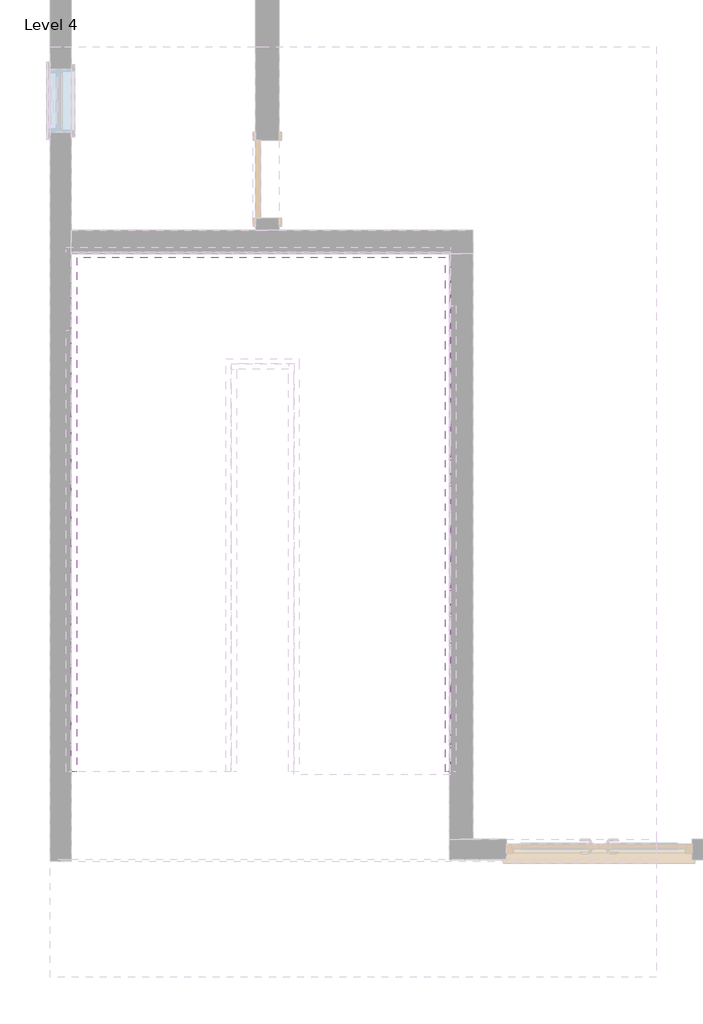
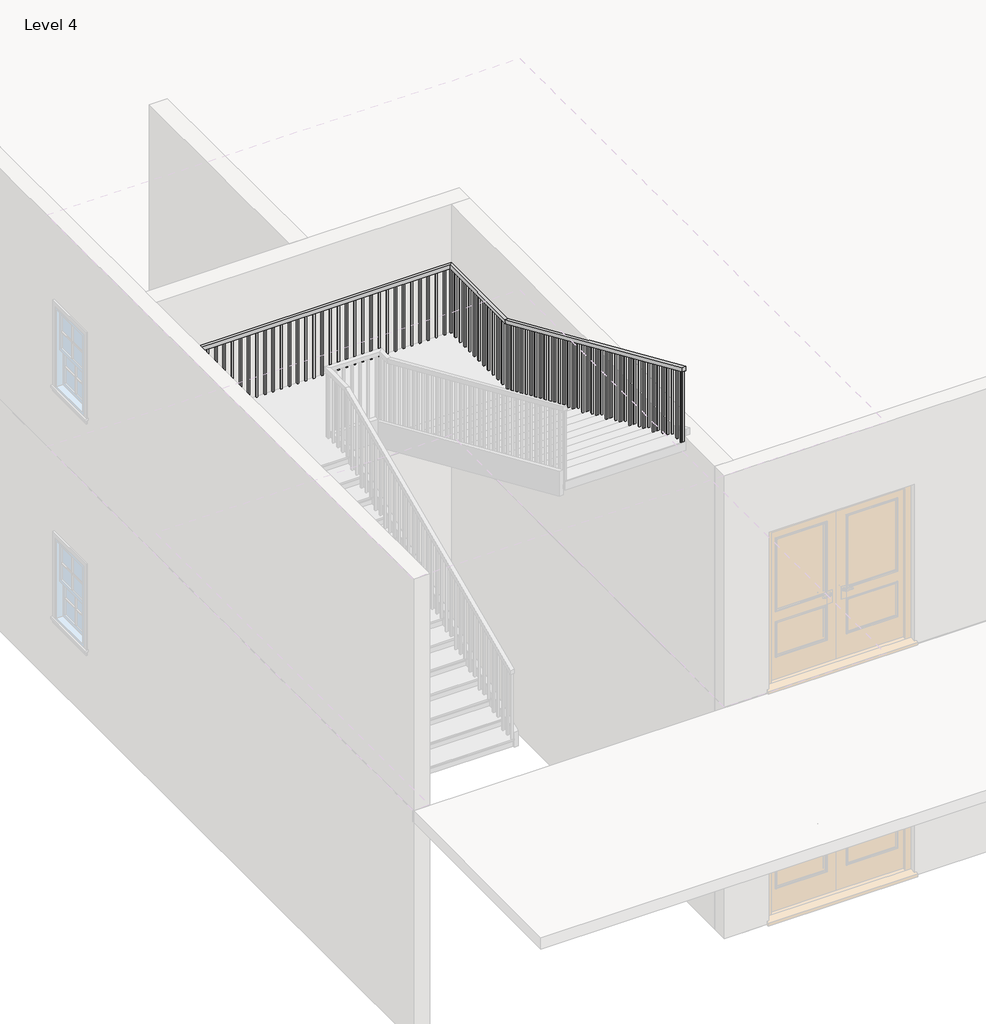
# One storey, part 4 of 5: 1 railing.
"""IFC4 building model written with IfcOpenShell, lengths in millimetres."""

from ifc_helpers import new_model, si_unit, frame, origin, place, context, project, spatial, polyline, outline, extrude, faceted_brep, element, save

model = new_model("IFC4")

# Units and contexts
model_context = context("Model", 3, world=origin())
ifc_project = project(units=[si_unit("LENGTHUNIT", "METRE", prefix="MILLI")], contexts=[model_context])

# Site, building, storey
site = spatial("IfcSite", under=ifc_project)
building = spatial("IfcBuilding", under=site)
storey = spatial("IfcBuildingStorey", under=building, Name="Level 4", Elevation=9144.0)

# Railing
placement = place(None, origin())
element("IfcRailing", 1, ObjectType="Handrail - Rectangular", at=placement, inside=storey, context=model_context, shape_type="SolidModel", body=[
    faceted_brep([(-7554.4415084, -6973.0610642, 12913.36), (-7554.4415084, -6973.0610642, 12857.8599828), (-7503.6415084, -6973.0610642, 12857.8599828), (-7503.6415084, -6973.0610642, 12913.36), (-7554.4415084, -3417.0610642, 14478.0), (-7554.4415084, -3406.3792071, 14427.2), (-7503.6415084, -3406.3792071, 14427.2), (-7503.6415084, -3417.0610642, 14478.0), (-7554.4415084, -1928.4217109, 14478.0), (-7554.4415084, -1928.4217109, 14427.2), (-7503.6415084, -1979.2217109, 14427.2), (-7503.6415084, -1979.2217109, 14478.0), (-3866.3290366, -1928.4217109, 14478.0), (-3866.3290366, -1928.4217109, 14427.2), (-3917.1290366, -1979.2217109, 14427.2), (-3917.1290366, -1979.2217109, 14478.0), (-3866.3290366, -3163.0610642, 14478.0), (-3866.3290366, -3173.7429214, 14427.2), (-3917.1290366, -3173.7429214, 14427.2), (-3917.1290366, -3163.0610642, 14478.0), (-3866.3290366, -6973.0610642, 16154.4), (-3917.1290366, -6973.0610642, 16154.4), (-3917.1290366, -6973.0610642, 16098.8999828), (-3866.3290366, -6973.0610642, 16098.8999828)], [[[0, 1, 2, 3]], [[1, 0, 4, 5]], [[2, 1, 5, 6]], [[3, 2, 6, 7]], [[0, 3, 7, 4]], [[5, 4, 8, 9]], [[6, 5, 9, 10]], [[7, 6, 10, 11]], [[4, 7, 11, 8]], [[9, 8, 12, 13]], [[10, 9, 13, 14]], [[11, 10, 14, 15]], [[8, 11, 15, 12]], [[13, 12, 16, 17]], [[14, 13, 17, 18]], [[15, 14, 18, 19]], [[12, 15, 19, 16]], [[20, 21, 22, 23]], [[17, 16, 20, 23]], [[18, 17, 23, 22]], [[19, 18, 22, 21]], [[16, 19, 21, 20]]]),
    extrude(outline(polyline([(-6922.6967109, 16076.7396674), (-6922.6967109, 15128.24), (-6941.7467109, 15128.24), (-6941.7467109, 16085.1216674), (-6922.6967109, 16076.7396674)])), frame((-3901.2540366, 0.0, 0.0), z_axis=(1.0, 0.0, 0.0), x_axis=(0.0, 1.0, 0.0)), (0.0, 0.0, 1.0), 19.05),
    extrude(outline(polyline([(-6821.0967109, 16032.0356674), (-6821.0967109, 15128.24), (-6840.1467109, 15128.24), (-6840.1467109, 16040.4176674), (-6821.0967109, 16032.0356674)])), frame((-3901.2540366, 0.0, 0.0), z_axis=(1.0, 0.0, 0.0), x_axis=(0.0, 1.0, 0.0)), (0.0, 0.0, 1.0), 19.05),
    extrude(outline(polyline([(-6719.4967109, 15987.3316674), (-6719.4967109, 15128.24), (-6738.5467109, 15128.24), (-6738.5467109, 15995.7136674), (-6719.4967109, 15987.3316674)])), frame((-3901.2540366, 0.0, 0.0), z_axis=(1.0, 0.0, 0.0), x_axis=(0.0, 1.0, 0.0)), (0.0, 0.0, 1.0), 19.05),
    extrude(outline(polyline([(-6617.8967109, 15942.6276674), (-6617.8967109, 15016.48), (-6636.9467109, 15016.48), (-6636.9467109, 15951.0096674), (-6617.8967109, 15942.6276674)])), frame((-3901.2540366, 0.0, 0.0), z_axis=(1.0, 0.0, 0.0), x_axis=(0.0, 1.0, 0.0)), (0.0, 0.0, 1.0), 19.05),
    extrude(outline(polyline([(-6516.2967109, 15897.9236674), (-6516.2967109, 15016.48), (-6535.3467109, 15016.48), (-6535.3467109, 15906.3056674), (-6516.2967109, 15897.9236674)])), frame((-3901.2540366, 0.0, 0.0), z_axis=(1.0, 0.0, 0.0), x_axis=(0.0, 1.0, 0.0)), (0.0, 0.0, 1.0), 19.05),
    extrude(outline(polyline([(-6414.6967109, 15853.2196674), (-6414.6967109, 14904.72), (-6433.7467109, 14904.72), (-6433.7467109, 15861.6016674), (-6414.6967109, 15853.2196674)])), frame((-3901.2540366, 0.0, 0.0), z_axis=(1.0, 0.0, 0.0), x_axis=(0.0, 1.0, 0.0)), (0.0, 0.0, 1.0), 19.05),
    extrude(outline(polyline([(-6313.0967109, 15808.5156674), (-6313.0967109, 14904.72), (-6332.1467109, 14904.72), (-6332.1467109, 15816.8976674), (-6313.0967109, 15808.5156674)])), frame((-3901.2540366, 0.0, 0.0), z_axis=(1.0, 0.0, 0.0), x_axis=(0.0, 1.0, 0.0)), (0.0, 0.0, 1.0), 19.05),
    extrude(outline(polyline([(-6211.4967109, 15763.8116674), (-6211.4967109, 14904.72), (-6230.5467109, 14904.72), (-6230.5467109, 15772.1936674), (-6211.4967109, 15763.8116674)])), frame((-3901.2540366, 0.0, 0.0), z_axis=(1.0, 0.0, 0.0), x_axis=(0.0, 1.0, 0.0)), (0.0, 0.0, 1.0), 19.05),
    extrude(outline(polyline([(-6109.8967109, 15719.1076674), (-6109.8967109, 14792.96), (-6128.9467109, 14792.96), (-6128.9467109, 15727.4896674), (-6109.8967109, 15719.1076674)])), frame((-3901.2540366, 0.0, 0.0), z_axis=(1.0, 0.0, 0.0), x_axis=(0.0, 1.0, 0.0)), (0.0, 0.0, 1.0), 19.05),
    extrude(outline(polyline([(-6008.2967109, 15674.4036674), (-6008.2967109, 14792.96), (-6027.3467109, 14792.96), (-6027.3467109, 15682.7856674), (-6008.2967109, 15674.4036674)])), frame((-3901.2540366, 0.0, 0.0), z_axis=(1.0, 0.0, 0.0), x_axis=(0.0, 1.0, 0.0)), (0.0, 0.0, 1.0), 19.05),
    extrude(outline(polyline([(-5906.6967109, 15629.6996674), (-5906.6967109, 14681.2), (-5925.7467109, 14681.2), (-5925.7467109, 15638.0816674), (-5906.6967109, 15629.6996674)])), frame((-3901.2540366, 0.0, 0.0), z_axis=(1.0, 0.0, 0.0), x_axis=(0.0, 1.0, 0.0)), (0.0, 0.0, 1.0), 19.05),
    extrude(outline(polyline([(-5805.0967109, 15584.9956674), (-5805.0967109, 14681.2), (-5824.1467109, 14681.2), (-5824.1467109, 15593.3776674), (-5805.0967109, 15584.9956674)])), frame((-3901.2540366, 0.0, 0.0), z_axis=(1.0, 0.0, 0.0), x_axis=(0.0, 1.0, 0.0)), (0.0, 0.0, 1.0), 19.05),
    extrude(outline(polyline([(-5703.4967109, 15540.2916674), (-5703.4967109, 14681.2), (-5722.5467109, 14681.2), (-5722.5467109, 15548.6736674), (-5703.4967109, 15540.2916674)])), frame((-3901.2540366, 0.0, 0.0), z_axis=(1.0, 0.0, 0.0), x_axis=(0.0, 1.0, 0.0)), (0.0, 0.0, 1.0), 19.05),
    extrude(outline(polyline([(-5601.8967109, 15495.5876674), (-5601.8967109, 14569.44), (-5620.9467109, 14569.44), (-5620.9467109, 15503.9696674), (-5601.8967109, 15495.5876674)])), frame((-3901.2540366, 0.0, 0.0), z_axis=(1.0, 0.0, 0.0), x_axis=(0.0, 1.0, 0.0)), (0.0, 0.0, 1.0), 19.05),
    extrude(outline(polyline([(-5500.2967109, 15450.8836674), (-5500.2967109, 14569.44), (-5519.3467109, 14569.44), (-5519.3467109, 15459.2656674), (-5500.2967109, 15450.8836674)])), frame((-3901.2540366, 0.0, 0.0), z_axis=(1.0, 0.0, 0.0), x_axis=(0.0, 1.0, 0.0)), (0.0, 0.0, 1.0), 19.05),
    extrude(outline(polyline([(-5398.6967109, 15406.1796674), (-5398.6967109, 14457.68), (-5417.7467109, 14457.68), (-5417.7467109, 15414.5616674), (-5398.6967109, 15406.1796674)])), frame((-3901.2540366, 0.0, 0.0), z_axis=(1.0, 0.0, 0.0), x_axis=(0.0, 1.0, 0.0)), (0.0, 0.0, 1.0), 19.05),
    extrude(outline(polyline([(-5297.0967109, 15361.4756674), (-5297.0967109, 14457.68), (-5316.1467109, 14457.68), (-5316.1467109, 15369.8576674), (-5297.0967109, 15361.4756674)])), frame((-3901.2540366, 0.0, 0.0), z_axis=(1.0, 0.0, 0.0), x_axis=(0.0, 1.0, 0.0)), (0.0, 0.0, 1.0), 19.05),
    extrude(outline(polyline([(-5195.4967109, 15316.7716674), (-5195.4967109, 14457.68), (-5214.5467109, 14457.68), (-5214.5467109, 15325.1536674), (-5195.4967109, 15316.7716674)])), frame((-3901.2540366, 0.0, 0.0), z_axis=(1.0, 0.0, 0.0), x_axis=(0.0, 1.0, 0.0)), (0.0, 0.0, 1.0), 19.05),
    extrude(outline(polyline([(-5093.8967109, 15272.0676674), (-5093.8967109, 14345.92), (-5112.9467109, 14345.92), (-5112.9467109, 15280.4496674), (-5093.8967109, 15272.0676674)])), frame((-3901.2540366, 0.0, 0.0), z_axis=(1.0, 0.0, 0.0), x_axis=(0.0, 1.0, 0.0)), (0.0, 0.0, 1.0), 19.05),
    extrude(outline(polyline([(-4992.2967109, 15227.3636674), (-4992.2967109, 14345.92), (-5011.3467109, 14345.92), (-5011.3467109, 15235.7456674), (-4992.2967109, 15227.3636674)])), frame((-3901.2540366, 0.0, 0.0), z_axis=(1.0, 0.0, 0.0), x_axis=(0.0, 1.0, 0.0)), (0.0, 0.0, 1.0), 19.05),
    extrude(outline(polyline([(-4890.6967109, 15182.6596674), (-4890.6967109, 14234.16), (-4909.7467109, 14234.16), (-4909.7467109, 15191.0416674), (-4890.6967109, 15182.6596674)])), frame((-3901.2540366, 0.0, 0.0), z_axis=(1.0, 0.0, 0.0), x_axis=(0.0, 1.0, 0.0)), (0.0, 0.0, 1.0), 19.05),
    extrude(outline(polyline([(-4789.0967109, 15137.9556674), (-4789.0967109, 14234.16), (-4808.1467109, 14234.16), (-4808.1467109, 15146.3376674), (-4789.0967109, 15137.9556674)])), frame((-3901.2540366, 0.0, 0.0), z_axis=(1.0, 0.0, 0.0), x_axis=(0.0, 1.0, 0.0)), (0.0, 0.0, 1.0), 19.05),
    extrude(outline(polyline([(-4687.4967109, 15093.2516674), (-4687.4967109, 14234.16), (-4706.5467109, 14234.16), (-4706.5467109, 15101.6336674), (-4687.4967109, 15093.2516674)])), frame((-3901.2540366, 0.0, 0.0), z_axis=(1.0, 0.0, 0.0), x_axis=(0.0, 1.0, 0.0)), (0.0, 0.0, 1.0), 19.05),
    extrude(outline(polyline([(-4585.8967109, 15048.5476674), (-4585.8967109, 14122.4), (-4604.9467109, 14122.4), (-4604.9467109, 15056.9296674), (-4585.8967109, 15048.5476674)])), frame((-3901.2540366, 0.0, 0.0), z_axis=(1.0, 0.0, 0.0), x_axis=(0.0, 1.0, 0.0)), (0.0, 0.0, 1.0), 19.05),
    extrude(outline(polyline([(-4484.2967109, 15003.8436674), (-4484.2967109, 14122.4), (-4503.3467109, 14122.4), (-4503.3467109, 15012.2256674), (-4484.2967109, 15003.8436674)])), frame((-3901.2540366, 0.0, 0.0), z_axis=(1.0, 0.0, 0.0), x_axis=(0.0, 1.0, 0.0)), (0.0, 0.0, 1.0), 19.05),
    extrude(outline(polyline([(-4382.6967109, 14959.1396674), (-4382.6967109, 14010.64), (-4401.7467109, 14010.64), (-4401.7467109, 14967.5216674), (-4382.6967109, 14959.1396674)])), frame((-3901.2540366, 0.0, 0.0), z_axis=(1.0, 0.0, 0.0), x_axis=(0.0, 1.0, 0.0)), (0.0, 0.0, 1.0), 19.05),
    extrude(outline(polyline([(-4281.0967109, 14914.4356674), (-4281.0967109, 14010.64), (-4300.1467109, 14010.64), (-4300.1467109, 14922.8176674), (-4281.0967109, 14914.4356674)])), frame((-3901.2540366, 0.0, 0.0), z_axis=(1.0, 0.0, 0.0), x_axis=(0.0, 1.0, 0.0)), (0.0, 0.0, 1.0), 19.05),
    extrude(outline(polyline([(-4179.4967109, 14869.7316674), (-4179.4967109, 14010.64), (-4198.5467109, 14010.64), (-4198.5467109, 14878.1136674), (-4179.4967109, 14869.7316674)])), frame((-3901.2540366, 0.0, 0.0), z_axis=(1.0, 0.0, 0.0), x_axis=(0.0, 1.0, 0.0)), (0.0, 0.0, 1.0), 19.05),
    extrude(outline(polyline([(-4077.8967109, 14825.0276674), (-4077.8967109, 13898.88), (-4096.9467109, 13898.88), (-4096.9467109, 14833.4096674), (-4077.8967109, 14825.0276674)])), frame((-3901.2540366, 0.0, 0.0), z_axis=(1.0, 0.0, 0.0), x_axis=(0.0, 1.0, 0.0)), (0.0, 0.0, 1.0), 19.05),
    extrude(outline(polyline([(-3976.2967109, 14780.3236674), (-3976.2967109, 13898.88), (-3995.3467109, 13898.88), (-3995.3467109, 14788.7056674), (-3976.2967109, 14780.3236674)])), frame((-3901.2540366, 0.0, 0.0), z_axis=(1.0, 0.0, 0.0), x_axis=(0.0, 1.0, 0.0)), (0.0, 0.0, 1.0), 19.05),
    extrude(outline(polyline([(-3874.6967109, 14735.6196674), (-3874.6967109, 13787.12), (-3893.7467109, 13787.12), (-3893.7467109, 14744.0016674), (-3874.6967109, 14735.6196674)])), frame((-3901.2540366, 0.0, 0.0), z_axis=(1.0, 0.0, 0.0), x_axis=(0.0, 1.0, 0.0)), (0.0, 0.0, 1.0), 19.05),
    extrude(outline(polyline([(-3773.0967109, 14690.9156674), (-3773.0967109, 13787.12), (-3792.1467109, 13787.12), (-3792.1467109, 14699.2976674), (-3773.0967109, 14690.9156674)])), frame((-3901.2540366, 0.0, 0.0), z_axis=(1.0, 0.0, 0.0), x_axis=(0.0, 1.0, 0.0)), (0.0, 0.0, 1.0), 19.05),
    extrude(outline(polyline([(-3671.4967109, 14646.2116674), (-3671.4967109, 13787.12), (-3690.5467109, 13787.12), (-3690.5467109, 14654.5936674), (-3671.4967109, 14646.2116674)])), frame((-3901.2540366, 0.0, 0.0), z_axis=(1.0, 0.0, 0.0), x_axis=(0.0, 1.0, 0.0)), (0.0, 0.0, 1.0), 19.05),
    extrude(outline(polyline([(-3569.8967109, 14601.5076674), (-3569.8967109, 13675.36), (-3588.9467109, 13675.36), (-3588.9467109, 14609.8896674), (-3569.8967109, 14601.5076674)])), frame((-3901.2540366, 0.0, 0.0), z_axis=(1.0, 0.0, 0.0), x_axis=(0.0, 1.0, 0.0)), (0.0, 0.0, 1.0), 19.05),
    extrude(outline(polyline([(-3468.2967109, 14556.8036674), (-3468.2967109, 13675.36), (-3487.3467109, 13675.36), (-3487.3467109, 14565.1856674), (-3468.2967109, 14556.8036674)])), frame((-3901.2540366, 0.0, 0.0), z_axis=(1.0, 0.0, 0.0), x_axis=(0.0, 1.0, 0.0)), (0.0, 0.0, 1.0), 19.05),
    extrude(outline(polyline([(-3366.6967109, 14512.0996674), (-3366.6967109, 13563.6), (-3385.7467109, 13563.6), (-3385.7467109, 14520.4816674), (-3366.6967109, 14512.0996674)])), frame((-3901.2540366, 0.0, 0.0), z_axis=(1.0, 0.0, 0.0), x_axis=(0.0, 1.0, 0.0)), (0.0, 0.0, 1.0), 19.05),
    extrude(outline(polyline([(-3265.0967109, 14467.3956674), (-3265.0967109, 13563.6), (-3284.1467109, 13563.6), (-3284.1467109, 14475.7776674), (-3265.0967109, 14467.3956674)])), frame((-3901.2540366, 0.0, 0.0), z_axis=(1.0, 0.0, 0.0), x_axis=(0.0, 1.0, 0.0)), (0.0, 0.0, 1.0), 19.05),
    extrude(outline(polyline([(-3163.4967109, 14422.6916674), (-3163.4967109, 13563.6), (-3182.5467109, 13563.6), (-3182.5467109, 14431.0736674), (-3163.4967109, 14422.6916674)])), frame((-3901.2540366, 0.0, 0.0), z_axis=(1.0, 0.0, 0.0), x_axis=(0.0, 1.0, 0.0)), (0.0, 0.0, 1.0), 19.05),
    extrude(outline(polyline([(-3882.2040366, -3061.8967109), (-3882.2040366, -3080.9467109), (-3901.2540366, -3080.9467109), (-3901.2540366, -3061.8967109), (-3882.2040366, -3061.8967109)])), frame((0.0, 0.0, 13563.6), z_axis=(0.0, 0.0, 1.0), x_axis=(1.0, 0.0, 0.0)), (0.0, 0.0, 1.0), 863.6),
    extrude(outline(polyline([(-3882.2040366, -2960.2967109), (-3882.2040366, -2979.3467109), (-3901.2540366, -2979.3467109), (-3901.2540366, -2960.2967109), (-3882.2040366, -2960.2967109)])), frame((0.0, 0.0, 13563.6), z_axis=(0.0, 0.0, 1.0), x_axis=(1.0, 0.0, 0.0)), (0.0, 0.0, 1.0), 863.6),
    extrude(outline(polyline([(-3882.2040366, -2858.6967109), (-3882.2040366, -2877.7467109), (-3901.2540366, -2877.7467109), (-3901.2540366, -2858.6967109), (-3882.2040366, -2858.6967109)])), frame((0.0, 0.0, 13563.6), z_axis=(0.0, 0.0, 1.0), x_axis=(1.0, 0.0, 0.0)), (0.0, 0.0, 1.0), 863.6),
    extrude(outline(polyline([(-3882.2040366, -2757.0967109), (-3882.2040366, -2776.1467109), (-3901.2540366, -2776.1467109), (-3901.2540366, -2757.0967109), (-3882.2040366, -2757.0967109)])), frame((0.0, 0.0, 13563.6), z_axis=(0.0, 0.0, 1.0), x_axis=(1.0, 0.0, 0.0)), (0.0, 0.0, 1.0), 863.6),
    extrude(outline(polyline([(-3882.2040366, -2655.4967109), (-3882.2040366, -2674.5467109), (-3901.2540366, -2674.5467109), (-3901.2540366, -2655.4967109), (-3882.2040366, -2655.4967109)])), frame((0.0, 0.0, 13563.6), z_axis=(0.0, 0.0, 1.0), x_axis=(1.0, 0.0, 0.0)), (0.0, 0.0, 1.0), 863.6),
    extrude(outline(polyline([(-3882.2040366, -2553.8967109), (-3882.2040366, -2572.9467109), (-3901.2540366, -2572.9467109), (-3901.2540366, -2553.8967109), (-3882.2040366, -2553.8967109)])), frame((0.0, 0.0, 13563.6), z_axis=(0.0, 0.0, 1.0), x_axis=(1.0, 0.0, 0.0)), (0.0, 0.0, 1.0), 863.6),
    extrude(outline(polyline([(-3882.2040366, -2452.2967109), (-3882.2040366, -2471.3467109), (-3901.2540366, -2471.3467109), (-3901.2540366, -2452.2967109), (-3882.2040366, -2452.2967109)])), frame((0.0, 0.0, 13563.6), z_axis=(0.0, 0.0, 1.0), x_axis=(1.0, 0.0, 0.0)), (0.0, 0.0, 1.0), 863.6),
    extrude(outline(polyline([(-3882.2040366, -2350.6967109), (-3882.2040366, -2369.7467109), (-3901.2540366, -2369.7467109), (-3901.2540366, -2350.6967109), (-3882.2040366, -2350.6967109)])), frame((0.0, 0.0, 13563.6), z_axis=(0.0, 0.0, 1.0), x_axis=(1.0, 0.0, 0.0)), (0.0, 0.0, 1.0), 863.6),
    extrude(outline(polyline([(-3882.2040366, -2249.0967109), (-3882.2040366, -2268.1467109), (-3901.2540366, -2268.1467109), (-3901.2540366, -2249.0967109), (-3882.2040366, -2249.0967109)])), frame((0.0, 0.0, 13563.6), z_axis=(0.0, 0.0, 1.0), x_axis=(1.0, 0.0, 0.0)), (0.0, 0.0, 1.0), 863.6),
    extrude(outline(polyline([(-3882.2040366, -2147.4967109), (-3882.2040366, -2166.5467109), (-3901.2540366, -2166.5467109), (-3901.2540366, -2147.4967109), (-3882.2040366, -2147.4967109)])), frame((0.0, 0.0, 13563.6), z_axis=(0.0, 0.0, 1.0), x_axis=(1.0, 0.0, 0.0)), (0.0, 0.0, 1.0), 863.6),
    extrude(outline(polyline([(-3882.2040366, -2045.8967109), (-3882.2040366, -2064.9467109), (-3901.2540366, -2064.9467109), (-3901.2540366, -2045.8967109), (-3882.2040366, -2045.8967109)])), frame((0.0, 0.0, 13563.6), z_axis=(0.0, 0.0, 1.0), x_axis=(1.0, 0.0, 0.0)), (0.0, 0.0, 1.0), 863.6),
    extrude(outline(polyline([(-3982.5665084, -1944.2967109), (-3963.5165084, -1944.2967109), (-3963.5165084, -1963.3467109), (-3982.5665084, -1963.3467109), (-3982.5665084, -1944.2967109)])), frame((0.0, 0.0, 13563.6), z_axis=(0.0, 0.0, 1.0), x_axis=(1.0, 0.0, 0.0)), (0.0, 0.0, 1.0), 863.6),
    extrude(outline(polyline([(-4084.1665084, -1944.2967109), (-4065.1165084, -1944.2967109), (-4065.1165084, -1963.3467109), (-4084.1665084, -1963.3467109), (-4084.1665084, -1944.2967109)])), frame((0.0, 0.0, 13563.6), z_axis=(0.0, 0.0, 1.0), x_axis=(1.0, 0.0, 0.0)), (0.0, 0.0, 1.0), 863.6),
    extrude(outline(polyline([(-4185.7665084, -1944.2967109), (-4166.7165084, -1944.2967109), (-4166.7165084, -1963.3467109), (-4185.7665084, -1963.3467109), (-4185.7665084, -1944.2967109)])), frame((0.0, 0.0, 13563.6), z_axis=(0.0, 0.0, 1.0), x_axis=(1.0, 0.0, 0.0)), (0.0, 0.0, 1.0), 863.6),
    extrude(outline(polyline([(-4287.3665084, -1944.2967109), (-4268.3165084, -1944.2967109), (-4268.3165084, -1963.3467109), (-4287.3665084, -1963.3467109), (-4287.3665084, -1944.2967109)])), frame((0.0, 0.0, 13563.6), z_axis=(0.0, 0.0, 1.0), x_axis=(1.0, 0.0, 0.0)), (0.0, 0.0, 1.0), 863.6),
    extrude(outline(polyline([(-4388.9665084, -1944.2967109), (-4369.9165084, -1944.2967109), (-4369.9165084, -1963.3467109), (-4388.9665084, -1963.3467109), (-4388.9665084, -1944.2967109)])), frame((0.0, 0.0, 13563.6), z_axis=(0.0, 0.0, 1.0), x_axis=(1.0, 0.0, 0.0)), (0.0, 0.0, 1.0), 863.6),
    extrude(outline(polyline([(-4490.5665084, -1944.2967109), (-4471.5165084, -1944.2967109), (-4471.5165084, -1963.3467109), (-4490.5665084, -1963.3467109), (-4490.5665084, -1944.2967109)])), frame((0.0, 0.0, 13563.6), z_axis=(0.0, 0.0, 1.0), x_axis=(1.0, 0.0, 0.0)), (0.0, 0.0, 1.0), 863.6),
    extrude(outline(polyline([(-4592.1665084, -1944.2967109), (-4573.1165084, -1944.2967109), (-4573.1165084, -1963.3467109), (-4592.1665084, -1963.3467109), (-4592.1665084, -1944.2967109)])), frame((0.0, 0.0, 13563.6), z_axis=(0.0, 0.0, 1.0), x_axis=(1.0, 0.0, 0.0)), (0.0, 0.0, 1.0), 863.6),
    extrude(outline(polyline([(-4693.7665084, -1944.2967109), (-4674.7165084, -1944.2967109), (-4674.7165084, -1963.3467109), (-4693.7665084, -1963.3467109), (-4693.7665084, -1944.2967109)])), frame((0.0, 0.0, 13563.6), z_axis=(0.0, 0.0, 1.0), x_axis=(1.0, 0.0, 0.0)), (0.0, 0.0, 1.0), 863.6),
    extrude(outline(polyline([(-4795.3665084, -1944.2967109), (-4776.3165084, -1944.2967109), (-4776.3165084, -1963.3467109), (-4795.3665084, -1963.3467109), (-4795.3665084, -1944.2967109)])), frame((0.0, 0.0, 13563.6), z_axis=(0.0, 0.0, 1.0), x_axis=(1.0, 0.0, 0.0)), (0.0, 0.0, 1.0), 863.6),
    extrude(outline(polyline([(-4896.9665084, -1944.2967109), (-4877.9165084, -1944.2967109), (-4877.9165084, -1963.3467109), (-4896.9665084, -1963.3467109), (-4896.9665084, -1944.2967109)])), frame((0.0, 0.0, 13563.6), z_axis=(0.0, 0.0, 1.0), x_axis=(1.0, 0.0, 0.0)), (0.0, 0.0, 1.0), 863.6),
    extrude(outline(polyline([(-4998.5665084, -1944.2967109), (-4979.5165084, -1944.2967109), (-4979.5165084, -1963.3467109), (-4998.5665084, -1963.3467109), (-4998.5665084, -1944.2967109)])), frame((0.0, 0.0, 13563.6), z_axis=(0.0, 0.0, 1.0), x_axis=(1.0, 0.0, 0.0)), (0.0, 0.0, 1.0), 863.6),
    extrude(outline(polyline([(-5100.1665084, -1944.2967109), (-5081.1165084, -1944.2967109), (-5081.1165084, -1963.3467109), (-5100.1665084, -1963.3467109), (-5100.1665084, -1944.2967109)])), frame((0.0, 0.0, 13563.6), z_axis=(0.0, 0.0, 1.0), x_axis=(1.0, 0.0, 0.0)), (0.0, 0.0, 1.0), 863.6),
    extrude(outline(polyline([(-5201.7665084, -1944.2967109), (-5182.7165084, -1944.2967109), (-5182.7165084, -1963.3467109), (-5201.7665084, -1963.3467109), (-5201.7665084, -1944.2967109)])), frame((0.0, 0.0, 13563.6), z_axis=(0.0, 0.0, 1.0), x_axis=(1.0, 0.0, 0.0)), (0.0, 0.0, 1.0), 863.6),
    extrude(outline(polyline([(-5303.3665084, -1944.2967109), (-5284.3165084, -1944.2967109), (-5284.3165084, -1963.3467109), (-5303.3665084, -1963.3467109), (-5303.3665084, -1944.2967109)])), frame((0.0, 0.0, 13563.6), z_axis=(0.0, 0.0, 1.0), x_axis=(1.0, 0.0, 0.0)), (0.0, 0.0, 1.0), 863.6),
    extrude(outline(polyline([(-5404.9665084, -1944.2967109), (-5385.9165084, -1944.2967109), (-5385.9165084, -1963.3467109), (-5404.9665084, -1963.3467109), (-5404.9665084, -1944.2967109)])), frame((0.0, 0.0, 13563.6), z_axis=(0.0, 0.0, 1.0), x_axis=(1.0, 0.0, 0.0)), (0.0, 0.0, 1.0), 863.6),
    extrude(outline(polyline([(-5506.5665084, -1944.2967109), (-5487.5165084, -1944.2967109), (-5487.5165084, -1963.3467109), (-5506.5665084, -1963.3467109), (-5506.5665084, -1944.2967109)])), frame((0.0, 0.0, 13563.6), z_axis=(0.0, 0.0, 1.0), x_axis=(1.0, 0.0, 0.0)), (0.0, 0.0, 1.0), 863.6),
    extrude(outline(polyline([(-5608.1665084, -1944.2967109), (-5589.1165084, -1944.2967109), (-5589.1165084, -1963.3467109), (-5608.1665084, -1963.3467109), (-5608.1665084, -1944.2967109)])), frame((0.0, 0.0, 13563.6), z_axis=(0.0, 0.0, 1.0), x_axis=(1.0, 0.0, 0.0)), (0.0, 0.0, 1.0), 863.6),
    extrude(outline(polyline([(-5709.7665084, -1944.2967109), (-5690.7165084, -1944.2967109), (-5690.7165084, -1963.3467109), (-5709.7665084, -1963.3467109), (-5709.7665084, -1944.2967109)])), frame((0.0, 0.0, 13563.6), z_axis=(0.0, 0.0, 1.0), x_axis=(1.0, 0.0, 0.0)), (0.0, 0.0, 1.0), 863.6),
    extrude(outline(polyline([(-5811.3665084, -1944.2967109), (-5792.3165084, -1944.2967109), (-5792.3165084, -1963.3467109), (-5811.3665084, -1963.3467109), (-5811.3665084, -1944.2967109)])), frame((0.0, 0.0, 13563.6), z_axis=(0.0, 0.0, 1.0), x_axis=(1.0, 0.0, 0.0)), (0.0, 0.0, 1.0), 863.6),
    extrude(outline(polyline([(-5912.9665084, -1944.2967109), (-5893.9165084, -1944.2967109), (-5893.9165084, -1963.3467109), (-5912.9665084, -1963.3467109), (-5912.9665084, -1944.2967109)])), frame((0.0, 0.0, 13563.6), z_axis=(0.0, 0.0, 1.0), x_axis=(1.0, 0.0, 0.0)), (0.0, 0.0, 1.0), 863.6),
    extrude(outline(polyline([(-6014.5665084, -1944.2967109), (-5995.5165084, -1944.2967109), (-5995.5165084, -1963.3467109), (-6014.5665084, -1963.3467109), (-6014.5665084, -1944.2967109)])), frame((0.0, 0.0, 13563.6), z_axis=(0.0, 0.0, 1.0), x_axis=(1.0, 0.0, 0.0)), (0.0, 0.0, 1.0), 863.6),
    extrude(outline(polyline([(-6116.1665084, -1944.2967109), (-6097.1165084, -1944.2967109), (-6097.1165084, -1963.3467109), (-6116.1665084, -1963.3467109), (-6116.1665084, -1944.2967109)])), frame((0.0, 0.0, 13563.6), z_axis=(0.0, 0.0, 1.0), x_axis=(1.0, 0.0, 0.0)), (0.0, 0.0, 1.0), 863.6),
    extrude(outline(polyline([(-6217.7665084, -1944.2967109), (-6198.7165084, -1944.2967109), (-6198.7165084, -1963.3467109), (-6217.7665084, -1963.3467109), (-6217.7665084, -1944.2967109)])), frame((0.0, 0.0, 13563.6), z_axis=(0.0, 0.0, 1.0), x_axis=(1.0, 0.0, 0.0)), (0.0, 0.0, 1.0), 863.6),
    extrude(outline(polyline([(-6319.3665084, -1944.2967109), (-6300.3165084, -1944.2967109), (-6300.3165084, -1963.3467109), (-6319.3665084, -1963.3467109), (-6319.3665084, -1944.2967109)])), frame((0.0, 0.0, 13563.6), z_axis=(0.0, 0.0, 1.0), x_axis=(1.0, 0.0, 0.0)), (0.0, 0.0, 1.0), 863.6),
    extrude(outline(polyline([(-6420.9665084, -1944.2967109), (-6401.9165084, -1944.2967109), (-6401.9165084, -1963.3467109), (-6420.9665084, -1963.3467109), (-6420.9665084, -1944.2967109)])), frame((0.0, 0.0, 13563.6), z_axis=(0.0, 0.0, 1.0), x_axis=(1.0, 0.0, 0.0)), (0.0, 0.0, 1.0), 863.6),
    extrude(outline(polyline([(-6522.5665084, -1944.2967109), (-6503.5165084, -1944.2967109), (-6503.5165084, -1963.3467109), (-6522.5665084, -1963.3467109), (-6522.5665084, -1944.2967109)])), frame((0.0, 0.0, 13563.6), z_axis=(0.0, 0.0, 1.0), x_axis=(1.0, 0.0, 0.0)), (0.0, 0.0, 1.0), 863.6),
    extrude(outline(polyline([(-6624.1665084, -1944.2967109), (-6605.1165084, -1944.2967109), (-6605.1165084, -1963.3467109), (-6624.1665084, -1963.3467109), (-6624.1665084, -1944.2967109)])), frame((0.0, 0.0, 13563.6), z_axis=(0.0, 0.0, 1.0), x_axis=(1.0, 0.0, 0.0)), (0.0, 0.0, 1.0), 863.6),
    extrude(outline(polyline([(-6725.7665084, -1944.2967109), (-6706.7165084, -1944.2967109), (-6706.7165084, -1963.3467109), (-6725.7665084, -1963.3467109), (-6725.7665084, -1944.2967109)])), frame((0.0, 0.0, 13563.6), z_axis=(0.0, 0.0, 1.0), x_axis=(1.0, 0.0, 0.0)), (0.0, 0.0, 1.0), 863.6),
    extrude(outline(polyline([(-6827.3665084, -1944.2967109), (-6808.3165084, -1944.2967109), (-6808.3165084, -1963.3467109), (-6827.3665084, -1963.3467109), (-6827.3665084, -1944.2967109)])), frame((0.0, 0.0, 13563.6), z_axis=(0.0, 0.0, 1.0), x_axis=(1.0, 0.0, 0.0)), (0.0, 0.0, 1.0), 863.6),
    extrude(outline(polyline([(-6928.9665084, -1944.2967109), (-6909.9165084, -1944.2967109), (-6909.9165084, -1963.3467109), (-6928.9665084, -1963.3467109), (-6928.9665084, -1944.2967109)])), frame((0.0, 0.0, 13563.6), z_axis=(0.0, 0.0, 1.0), x_axis=(1.0, 0.0, 0.0)), (0.0, 0.0, 1.0), 863.6),
    extrude(outline(polyline([(-7030.5665084, -1944.2967109), (-7011.5165084, -1944.2967109), (-7011.5165084, -1963.3467109), (-7030.5665084, -1963.3467109), (-7030.5665084, -1944.2967109)])), frame((0.0, 0.0, 13563.6), z_axis=(0.0, 0.0, 1.0), x_axis=(1.0, 0.0, 0.0)), (0.0, 0.0, 1.0), 863.6),
    extrude(outline(polyline([(-7132.1665084, -1944.2967109), (-7113.1165084, -1944.2967109), (-7113.1165084, -1963.3467109), (-7132.1665084, -1963.3467109), (-7132.1665084, -1944.2967109)])), frame((0.0, 0.0, 13563.6), z_axis=(0.0, 0.0, 1.0), x_axis=(1.0, 0.0, 0.0)), (0.0, 0.0, 1.0), 863.6),
    extrude(outline(polyline([(-7233.7665084, -1944.2967109), (-7214.7165084, -1944.2967109), (-7214.7165084, -1963.3467109), (-7233.7665084, -1963.3467109), (-7233.7665084, -1944.2967109)])), frame((0.0, 0.0, 13563.6), z_axis=(0.0, 0.0, 1.0), x_axis=(1.0, 0.0, 0.0)), (0.0, 0.0, 1.0), 863.6),
    extrude(outline(polyline([(-7335.3665084, -1944.2967109), (-7316.3165084, -1944.2967109), (-7316.3165084, -1963.3467109), (-7335.3665084, -1963.3467109), (-7335.3665084, -1944.2967109)])), frame((0.0, 0.0, 13563.6), z_axis=(0.0, 0.0, 1.0), x_axis=(1.0, 0.0, 0.0)), (0.0, 0.0, 1.0), 863.6),
    extrude(outline(polyline([(-7436.9665084, -1944.2967109), (-7417.9165084, -1944.2967109), (-7417.9165084, -1963.3467109), (-7436.9665084, -1963.3467109), (-7436.9665084, -1944.2967109)])), frame((0.0, 0.0, 13563.6), z_axis=(0.0, 0.0, 1.0), x_axis=(1.0, 0.0, 0.0)), (0.0, 0.0, 1.0), 863.6),
    extrude(outline(polyline([(-7538.5665084, -2004.1860642), (-7538.5665084, -1985.1360642), (-7519.5165084, -1985.1360642), (-7519.5165084, -2004.1860642), (-7538.5665084, -2004.1860642)])), frame((0.0, 0.0, 13563.6), z_axis=(0.0, 0.0, 1.0), x_axis=(1.0, 0.0, 0.0)), (0.0, 0.0, 1.0), 863.6),
    extrude(outline(polyline([(-7538.5665084, -2105.7860642), (-7538.5665084, -2086.7360642), (-7519.5165084, -2086.7360642), (-7519.5165084, -2105.7860642), (-7538.5665084, -2105.7860642)])), frame((0.0, 0.0, 13563.6), z_axis=(0.0, 0.0, 1.0), x_axis=(1.0, 0.0, 0.0)), (0.0, 0.0, 1.0), 863.6),
    extrude(outline(polyline([(-7538.5665084, -2207.3860642), (-7538.5665084, -2188.3360642), (-7519.5165084, -2188.3360642), (-7519.5165084, -2207.3860642), (-7538.5665084, -2207.3860642)])), frame((0.0, 0.0, 13563.6), z_axis=(0.0, 0.0, 1.0), x_axis=(1.0, 0.0, 0.0)), (0.0, 0.0, 1.0), 863.6),
    extrude(outline(polyline([(-7538.5665084, -2308.9860642), (-7538.5665084, -2289.9360642), (-7519.5165084, -2289.9360642), (-7519.5165084, -2308.9860642), (-7538.5665084, -2308.9860642)])), frame((0.0, 0.0, 13563.6), z_axis=(0.0, 0.0, 1.0), x_axis=(1.0, 0.0, 0.0)), (0.0, 0.0, 1.0), 863.6),
    extrude(outline(polyline([(-7538.5665084, -2410.5860642), (-7538.5665084, -2391.5360642), (-7519.5165084, -2391.5360642), (-7519.5165084, -2410.5860642), (-7538.5665084, -2410.5860642)])), frame((0.0, 0.0, 13563.6), z_axis=(0.0, 0.0, 1.0), x_axis=(1.0, 0.0, 0.0)), (0.0, 0.0, 1.0), 863.6),
    extrude(outline(polyline([(-7538.5665084, -2512.1860642), (-7538.5665084, -2493.1360642), (-7519.5165084, -2493.1360642), (-7519.5165084, -2512.1860642), (-7538.5665084, -2512.1860642)])), frame((0.0, 0.0, 13563.6), z_axis=(0.0, 0.0, 1.0), x_axis=(1.0, 0.0, 0.0)), (0.0, 0.0, 1.0), 863.6),
    extrude(outline(polyline([(-7538.5665084, -2613.7860642), (-7538.5665084, -2594.7360642), (-7519.5165084, -2594.7360642), (-7519.5165084, -2613.7860642), (-7538.5665084, -2613.7860642)])), frame((0.0, 0.0, 13563.6), z_axis=(0.0, 0.0, 1.0), x_axis=(1.0, 0.0, 0.0)), (0.0, 0.0, 1.0), 863.6),
    extrude(outline(polyline([(-7538.5665084, -2715.3860642), (-7538.5665084, -2696.3360642), (-7519.5165084, -2696.3360642), (-7519.5165084, -2715.3860642), (-7538.5665084, -2715.3860642)])), frame((0.0, 0.0, 13563.6), z_axis=(0.0, 0.0, 1.0), x_axis=(1.0, 0.0, 0.0)), (0.0, 0.0, 1.0), 863.6),
    extrude(outline(polyline([(-7538.5665084, -2816.9860642), (-7538.5665084, -2797.9360642), (-7519.5165084, -2797.9360642), (-7519.5165084, -2816.9860642), (-7538.5665084, -2816.9860642)])), frame((0.0, 0.0, 13563.6), z_axis=(0.0, 0.0, 1.0), x_axis=(1.0, 0.0, 0.0)), (0.0, 0.0, 1.0), 863.6),
    extrude(outline(polyline([(-7538.5665084, -2918.5860642), (-7538.5665084, -2899.5360642), (-7519.5165084, -2899.5360642), (-7519.5165084, -2918.5860642), (-7538.5665084, -2918.5860642)])), frame((0.0, 0.0, 13563.6), z_axis=(0.0, 0.0, 1.0), x_axis=(1.0, 0.0, 0.0)), (0.0, 0.0, 1.0), 863.6),
    extrude(outline(polyline([(-7538.5665084, -3020.1860642), (-7538.5665084, -3001.1360642), (-7519.5165084, -3001.1360642), (-7519.5165084, -3020.1860642), (-7538.5665084, -3020.1860642)])), frame((0.0, 0.0, 13563.6), z_axis=(0.0, 0.0, 1.0), x_axis=(1.0, 0.0, 0.0)), (0.0, 0.0, 1.0), 863.6),
    extrude(outline(polyline([(-7538.5665084, -3121.7860642), (-7538.5665084, -3102.7360642), (-7519.5165084, -3102.7360642), (-7519.5165084, -3121.7860642), (-7538.5665084, -3121.7860642)])), frame((0.0, 0.0, 13563.6), z_axis=(0.0, 0.0, 1.0), x_axis=(1.0, 0.0, 0.0)), (0.0, 0.0, 1.0), 863.6),
    extrude(outline(polyline([(-7538.5665084, -3223.3860642), (-7538.5665084, -3204.3360642), (-7519.5165084, -3204.3360642), (-7519.5165084, -3223.3860642), (-7538.5665084, -3223.3860642)])), frame((0.0, 0.0, 13563.6), z_axis=(0.0, 0.0, 1.0), x_axis=(1.0, 0.0, 0.0)), (0.0, 0.0, 1.0), 863.6),
    extrude(outline(polyline([(-7538.5665084, -3324.9860642), (-7538.5665084, -3305.9360642), (-7519.5165084, -3305.9360642), (-7519.5165084, -3324.9860642), (-7538.5665084, -3324.9860642)])), frame((0.0, 0.0, 13563.6), z_axis=(0.0, 0.0, 1.0), x_axis=(1.0, 0.0, 0.0)), (0.0, 0.0, 1.0), 863.6),
    extrude(outline(polyline([(-3407.5360642, 14426.6909828), (-3407.5360642, 13563.6), (-3426.5860642, 13563.6), (-3426.5860642, 14418.3089828), (-3407.5360642, 14426.6909828)])), frame((-7538.5665084, 0.0, 0.0), z_axis=(1.0, 0.0, 0.0), x_axis=(0.0, 1.0, 0.0)), (0.0, 0.0, 1.0), 19.05),
    extrude(outline(polyline([(-3509.1360642, 14381.9869828), (-3509.1360642, 13451.84), (-3528.1860642, 13451.84), (-3528.1860642, 14373.6049828), (-3509.1360642, 14381.9869828)])), frame((-7538.5665084, 0.0, 0.0), z_axis=(1.0, 0.0, 0.0), x_axis=(0.0, 1.0, 0.0)), (0.0, 0.0, 1.0), 19.05),
    extrude(outline(polyline([(-3610.7360642, 14337.2829828), (-3610.7360642, 13451.84), (-3629.7860642, 13451.84), (-3629.7860642, 14328.9009828), (-3610.7360642, 14337.2829828)])), frame((-7538.5665084, 0.0, 0.0), z_axis=(1.0, 0.0, 0.0), x_axis=(0.0, 1.0, 0.0)), (0.0, 0.0, 1.0), 19.05),
    extrude(outline(polyline([(-3712.3360642, 14292.5789828), (-3712.3360642, 13340.08), (-3731.3860642, 13340.08), (-3731.3860642, 14284.1969828), (-3712.3360642, 14292.5789828)])), frame((-7538.5665084, 0.0, 0.0), z_axis=(1.0, 0.0, 0.0), x_axis=(0.0, 1.0, 0.0)), (0.0, 0.0, 1.0), 19.05),
    extrude(outline(polyline([(-3813.9360642, 14247.8749828), (-3813.9360642, 13340.08), (-3832.9860642, 13340.08), (-3832.9860642, 14239.4929828), (-3813.9360642, 14247.8749828)])), frame((-7538.5665084, 0.0, 0.0), z_axis=(1.0, 0.0, 0.0), x_axis=(0.0, 1.0, 0.0)), (0.0, 0.0, 1.0), 19.05),
    extrude(outline(polyline([(-3915.5360642, 14203.1709828), (-3915.5360642, 13340.08), (-3934.5860642, 13340.08), (-3934.5860642, 14194.7889828), (-3915.5360642, 14203.1709828)])), frame((-7538.5665084, 0.0, 0.0), z_axis=(1.0, 0.0, 0.0), x_axis=(0.0, 1.0, 0.0)), (0.0, 0.0, 1.0), 19.05),
    extrude(outline(polyline([(-4017.1360642, 14158.4669828), (-4017.1360642, 13228.32), (-4036.1860642, 13228.32), (-4036.1860642, 14150.0849828), (-4017.1360642, 14158.4669828)])), frame((-7538.5665084, 0.0, 0.0), z_axis=(1.0, 0.0, 0.0), x_axis=(0.0, 1.0, 0.0)), (0.0, 0.0, 1.0), 19.05),
    extrude(outline(polyline([(-4118.7360642, 14113.7629828), (-4118.7360642, 13228.32), (-4137.7860642, 13228.32), (-4137.7860642, 14105.3809828), (-4118.7360642, 14113.7629828)])), frame((-7538.5665084, 0.0, 0.0), z_axis=(1.0, 0.0, 0.0), x_axis=(0.0, 1.0, 0.0)), (0.0, 0.0, 1.0), 19.05),
    extrude(outline(polyline([(-4220.3360642, 14069.0589828), (-4220.3360642, 13116.56), (-4239.3860642, 13116.56), (-4239.3860642, 14060.6769828), (-4220.3360642, 14069.0589828)])), frame((-7538.5665084, 0.0, 0.0), z_axis=(1.0, 0.0, 0.0), x_axis=(0.0, 1.0, 0.0)), (0.0, 0.0, 1.0), 19.05),
    extrude(outline(polyline([(-4321.9360642, 14024.3549828), (-4321.9360642, 13116.56), (-4340.9860642, 13116.56), (-4340.9860642, 14015.9729828), (-4321.9360642, 14024.3549828)])), frame((-7538.5665084, 0.0, 0.0), z_axis=(1.0, 0.0, 0.0), x_axis=(0.0, 1.0, 0.0)), (0.0, 0.0, 1.0), 19.05),
    extrude(outline(polyline([(-4423.5360642, 13979.6509828), (-4423.5360642, 13116.56), (-4442.5860642, 13116.56), (-4442.5860642, 13971.2689828), (-4423.5360642, 13979.6509828)])), frame((-7538.5665084, 0.0, 0.0), z_axis=(1.0, 0.0, 0.0), x_axis=(0.0, 1.0, 0.0)), (0.0, 0.0, 1.0), 19.05),
    extrude(outline(polyline([(-4525.1360642, 13934.9469828), (-4525.1360642, 13004.8), (-4544.1860642, 13004.8), (-4544.1860642, 13926.5649828), (-4525.1360642, 13934.9469828)])), frame((-7538.5665084, 0.0, 0.0), z_axis=(1.0, 0.0, 0.0), x_axis=(0.0, 1.0, 0.0)), (0.0, 0.0, 1.0), 19.05),
    extrude(outline(polyline([(-4626.7360642, 13890.2429828), (-4626.7360642, 13004.8), (-4645.7860642, 13004.8), (-4645.7860642, 13881.8609828), (-4626.7360642, 13890.2429828)])), frame((-7538.5665084, 0.0, 0.0), z_axis=(1.0, 0.0, 0.0), x_axis=(0.0, 1.0, 0.0)), (0.0, 0.0, 1.0), 19.05),
    extrude(outline(polyline([(-4728.3360642, 13845.5389828), (-4728.3360642, 12893.04), (-4747.3860642, 12893.04), (-4747.3860642, 13837.1569828), (-4728.3360642, 13845.5389828)])), frame((-7538.5665084, 0.0, 0.0), z_axis=(1.0, 0.0, 0.0), x_axis=(0.0, 1.0, 0.0)), (0.0, 0.0, 1.0), 19.05),
    extrude(outline(polyline([(-4829.9360642, 13800.8349828), (-4829.9360642, 12893.04), (-4848.9860642, 12893.04), (-4848.9860642, 13792.4529828), (-4829.9360642, 13800.8349828)])), frame((-7538.5665084, 0.0, 0.0), z_axis=(1.0, 0.0, 0.0), x_axis=(0.0, 1.0, 0.0)), (0.0, 0.0, 1.0), 19.05),
    extrude(outline(polyline([(-4931.5360642, 13756.1309828), (-4931.5360642, 12893.04), (-4950.5860642, 12893.04), (-4950.5860642, 13747.7489828), (-4931.5360642, 13756.1309828)])), frame((-7538.5665084, 0.0, 0.0), z_axis=(1.0, 0.0, 0.0), x_axis=(0.0, 1.0, 0.0)), (0.0, 0.0, 1.0), 19.05),
    extrude(outline(polyline([(-5033.1360642, 13711.4269828), (-5033.1360642, 12781.28), (-5052.1860642, 12781.28), (-5052.1860642, 13703.0449828), (-5033.1360642, 13711.4269828)])), frame((-7538.5665084, 0.0, 0.0), z_axis=(1.0, 0.0, 0.0), x_axis=(0.0, 1.0, 0.0)), (0.0, 0.0, 1.0), 19.05),
    extrude(outline(polyline([(-5134.7360642, 13666.7229828), (-5134.7360642, 12781.28), (-5153.7860642, 12781.28), (-5153.7860642, 13658.3409828), (-5134.7360642, 13666.7229828)])), frame((-7538.5665084, 0.0, 0.0), z_axis=(1.0, 0.0, 0.0), x_axis=(0.0, 1.0, 0.0)), (0.0, 0.0, 1.0), 19.05),
    extrude(outline(polyline([(-5236.3360642, 13622.0189828), (-5236.3360642, 12669.52), (-5255.3860642, 12669.52), (-5255.3860642, 13613.6369828), (-5236.3360642, 13622.0189828)])), frame((-7538.5665084, 0.0, 0.0), z_axis=(1.0, 0.0, 0.0), x_axis=(0.0, 1.0, 0.0)), (0.0, 0.0, 1.0), 19.05),
    extrude(outline(polyline([(-5337.9360642, 13577.3149828), (-5337.9360642, 12669.52), (-5356.9860642, 12669.52), (-5356.9860642, 13568.9329828), (-5337.9360642, 13577.3149828)])), frame((-7538.5665084, 0.0, 0.0), z_axis=(1.0, 0.0, 0.0), x_axis=(0.0, 1.0, 0.0)), (0.0, 0.0, 1.0), 19.05),
    extrude(outline(polyline([(-5439.5360642, 13532.6109828), (-5439.5360642, 12669.52), (-5458.5860642, 12669.52), (-5458.5860642, 13524.2289828), (-5439.5360642, 13532.6109828)])), frame((-7538.5665084, 0.0, 0.0), z_axis=(1.0, 0.0, 0.0), x_axis=(0.0, 1.0, 0.0)), (0.0, 0.0, 1.0), 19.05),
    extrude(outline(polyline([(-5541.1360642, 13487.9069828), (-5541.1360642, 12557.76), (-5560.1860642, 12557.76), (-5560.1860642, 13479.5249828), (-5541.1360642, 13487.9069828)])), frame((-7538.5665084, 0.0, 0.0), z_axis=(1.0, 0.0, 0.0), x_axis=(0.0, 1.0, 0.0)), (0.0, 0.0, 1.0), 19.05),
    extrude(outline(polyline([(-5642.7360642, 13443.2029828), (-5642.7360642, 12557.76), (-5661.7860642, 12557.76), (-5661.7860642, 13434.8209828), (-5642.7360642, 13443.2029828)])), frame((-7538.5665084, 0.0, 0.0), z_axis=(1.0, 0.0, 0.0), x_axis=(0.0, 1.0, 0.0)), (0.0, 0.0, 1.0), 19.05),
    extrude(outline(polyline([(-5744.3360642, 13398.4989828), (-5744.3360642, 12446.0), (-5763.3860642, 12446.0), (-5763.3860642, 13390.1169828), (-5744.3360642, 13398.4989828)])), frame((-7538.5665084, 0.0, 0.0), z_axis=(1.0, 0.0, 0.0), x_axis=(0.0, 1.0, 0.0)), (0.0, 0.0, 1.0), 19.05),
    extrude(outline(polyline([(-5845.9360642, 13353.7949828), (-5845.9360642, 12446.0), (-5864.9860642, 12446.0), (-5864.9860642, 13345.4129828), (-5845.9360642, 13353.7949828)])), frame((-7538.5665084, 0.0, 0.0), z_axis=(1.0, 0.0, 0.0), x_axis=(0.0, 1.0, 0.0)), (0.0, 0.0, 1.0), 19.05),
    extrude(outline(polyline([(-5947.5360642, 13309.0909828), (-5947.5360642, 12446.0), (-5966.5860642, 12446.0), (-5966.5860642, 13300.7089828), (-5947.5360642, 13309.0909828)])), frame((-7538.5665084, 0.0, 0.0), z_axis=(1.0, 0.0, 0.0), x_axis=(0.0, 1.0, 0.0)), (0.0, 0.0, 1.0), 19.05),
    extrude(outline(polyline([(-6049.1360642, 13264.3869828), (-6049.1360642, 12334.24), (-6068.1860642, 12334.24), (-6068.1860642, 13256.0049828), (-6049.1360642, 13264.3869828)])), frame((-7538.5665084, 0.0, 0.0), z_axis=(1.0, 0.0, 0.0), x_axis=(0.0, 1.0, 0.0)), (0.0, 0.0, 1.0), 19.05),
    extrude(outline(polyline([(-6150.7360642, 13219.6829828), (-6150.7360642, 12334.24), (-6169.7860642, 12334.24), (-6169.7860642, 13211.3009828), (-6150.7360642, 13219.6829828)])), frame((-7538.5665084, 0.0, 0.0), z_axis=(1.0, 0.0, 0.0), x_axis=(0.0, 1.0, 0.0)), (0.0, 0.0, 1.0), 19.05),
    extrude(outline(polyline([(-6252.3360642, 13174.9789828), (-6252.3360642, 12222.48), (-6271.3860642, 12222.48), (-6271.3860642, 13166.5969828), (-6252.3360642, 13174.9789828)])), frame((-7538.5665084, 0.0, 0.0), z_axis=(1.0, 0.0, 0.0), x_axis=(0.0, 1.0, 0.0)), (0.0, 0.0, 1.0), 19.05),
    extrude(outline(polyline([(-6353.9360642, 13130.2749828), (-6353.9360642, 12222.48), (-6372.9860642, 12222.48), (-6372.9860642, 13121.8929828), (-6353.9360642, 13130.2749828)])), frame((-7538.5665084, 0.0, 0.0), z_axis=(1.0, 0.0, 0.0), x_axis=(0.0, 1.0, 0.0)), (0.0, 0.0, 1.0), 19.05),
    extrude(outline(polyline([(-6455.5360642, 13085.5709828), (-6455.5360642, 12222.48), (-6474.5860642, 12222.48), (-6474.5860642, 13077.1889828), (-6455.5360642, 13085.5709828)])), frame((-7538.5665084, 0.0, 0.0), z_axis=(1.0, 0.0, 0.0), x_axis=(0.0, 1.0, 0.0)), (0.0, 0.0, 1.0), 19.05),
    extrude(outline(polyline([(-6557.1360642, 13040.8669828), (-6557.1360642, 12110.72), (-6576.1860642, 12110.72), (-6576.1860642, 13032.4849828), (-6557.1360642, 13040.8669828)])), frame((-7538.5665084, 0.0, 0.0), z_axis=(1.0, 0.0, 0.0), x_axis=(0.0, 1.0, 0.0)), (0.0, 0.0, 1.0), 19.05),
    extrude(outline(polyline([(-6658.7360642, 12996.1629828), (-6658.7360642, 12110.72), (-6677.7860642, 12110.72), (-6677.7860642, 12987.7809828), (-6658.7360642, 12996.1629828)])), frame((-7538.5665084, 0.0, 0.0), z_axis=(1.0, 0.0, 0.0), x_axis=(0.0, 1.0, 0.0)), (0.0, 0.0, 1.0), 19.05),
    extrude(outline(polyline([(-6760.3360642, 12951.4589828), (-6760.3360642, 11998.96), (-6779.3860642, 11998.96), (-6779.3860642, 12943.0769828), (-6760.3360642, 12951.4589828)])), frame((-7538.5665084, 0.0, 0.0), z_axis=(1.0, 0.0, 0.0), x_axis=(0.0, 1.0, 0.0)), (0.0, 0.0, 1.0), 19.05),
    extrude(outline(polyline([(-6861.9360642, 12906.7549828), (-6861.9360642, 11998.96), (-6880.9860642, 11998.96), (-6880.9860642, 12898.3729828), (-6861.9360642, 12906.7549828)])), frame((-7538.5665084, 0.0, 0.0), z_axis=(1.0, 0.0, 0.0), x_axis=(0.0, 1.0, 0.0)), (0.0, 0.0, 1.0), 19.05),
    extrude(outline(polyline([(-3901.2540366, -1944.2967109), (-3882.2040366, -1944.2967109), (-3882.2040366, -1963.3467109), (-3901.2540366, -1963.3467109), (-3901.2540366, -1944.2967109)])), frame((0.0, 0.0, 13563.6), z_axis=(0.0, 0.0, 1.0), x_axis=(1.0, 0.0, 0.0)), (0.0, 0.0, 1.0), 863.6),
    extrude(outline(polyline([(-7538.5665084, -1963.3467109), (-7538.5665084, -1944.2967109), (-7519.5165084, -1944.2967109), (-7519.5165084, -1963.3467109), (-7538.5665084, -1963.3467109)])), frame((0.0, 0.0, 13563.6), z_axis=(0.0, 0.0, 1.0), x_axis=(1.0, 0.0, 0.0)), (0.0, 0.0, 1.0), 863.6),
    extrude(outline(polyline([(-6954.0110642, 16090.5179828), (-6954.0110642, 15128.24), (-6973.0610642, 15128.24), (-6973.0610642, 16098.8999828), (-6954.0110642, 16090.5179828)])), frame((-3901.2540366, 0.0, 0.0), z_axis=(1.0, 0.0, 0.0), x_axis=(0.0, 1.0, 0.0)), (0.0, 0.0, 1.0), 19.05),
    extrude(outline(polyline([(-6954.0110642, 12866.2419828), (-6954.0110642, 11998.96), (-6973.0610642, 11998.96), (-6973.0610642, 12857.8599828), (-6954.0110642, 12866.2419828)])), frame((-7538.5665084, 0.0, 0.0), z_axis=(1.0, 0.0, 0.0), x_axis=(0.0, 1.0, 0.0)), (0.0, 0.0, 1.0), 19.05),
])

save(model, "model.ifc")

# Revit data of these elements
# Type "Handrail - Rectangular"
#   Assembly Code = "C2010400"
#   built-in parameter 1008612 = 0.0416667 (stored number, unit not read)
#   built-in parameter 1008611 = 0.0416667 (stored number, unit not read)
#   built-in parameter 1008609 = 0.333333 (stored number, unit not read)
#   built-in parameter 1008604 = 0.166667 (stored number, unit not read)
#   built-in parameter 1008603 = 0.166667 (stored number, unit not read)
#   Railing Height = 3' - 0"
#   built-in parameter 1008630 = 2
#   built-in parameter 1008610 = 2
#   built-in parameter 1008618 = Baluster - Square : 3/4"
# Element 1 (IfcRailing, "Handrail - Rectangular")
#   Phase Created = New Construction
